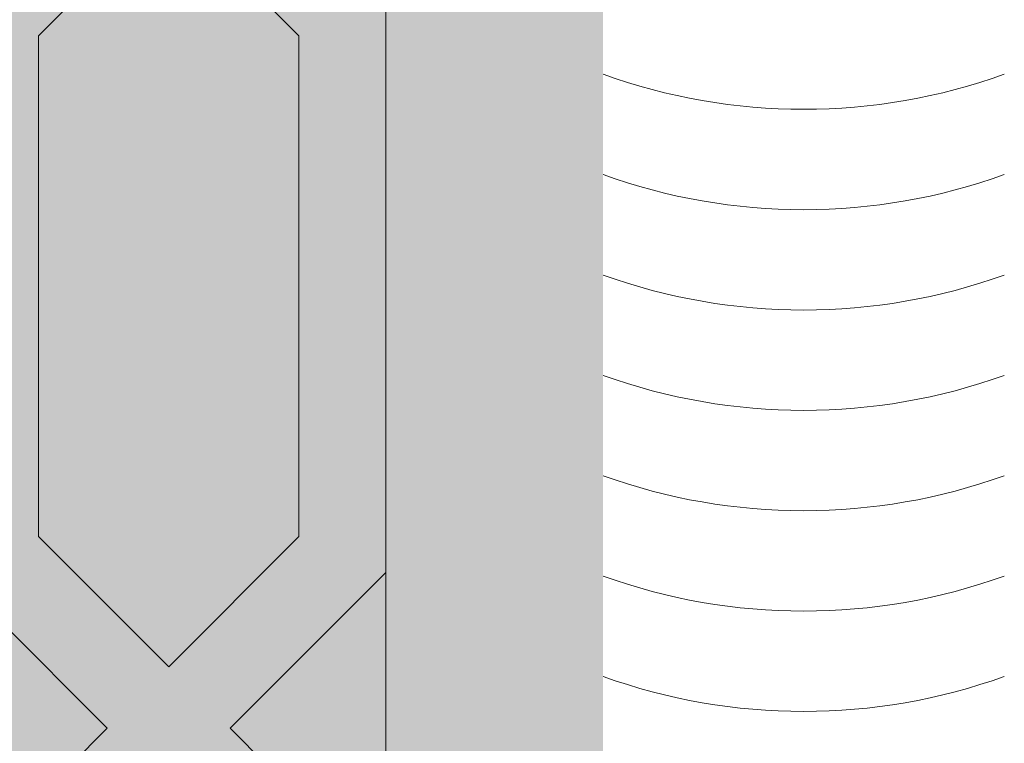
# Model space of a CAD drawing. Units: inches. Extents: x 844 to 2234, y 346 to 1084.
# Tile 38 of 93: x 1262.676 to 1265.567, y 699.229 to 701.353. Entities that reach past the tile are written whole.
import ezdxf

# ---------------------------------------------------------------- set-up
doc = ezdxf.new("R2010")
doc.units = ezdxf.units.IN
doc.header["$MEASUREMENT"] = 0
doc.layers.add('furniture', color=8, linetype='Continuous', lineweight=18)
doc.layers.add('RA-AP-01$0$INT', color=35, linetype='Continuous', lineweight=5)
doc.layers.add('RA-AP-01$0$FURN', color=3, linetype='Continuous')

# ---------------------------------------------------------------- blocks, each defined once
blk = doc.blocks.new('A$C18D01794')
at = {"layer": 'RA-AP-01$0$INT'}
h = blk.add_hatch(color=256, dxfattribs=at)
h.paths.add_polyline_path([(4.355206456958071, -6.156712009588037), (4.355206456958071, -8.056712009588038), (5.455206456958072, -8.056712009588038), (5.455206456958072, -6.156712009588037)])
h.paths.add_polyline_path([(4.405206456958072, -8.006712009588039), (4.405206456958072, -6.206712009588038), (5.405206456958072, -6.206712009588038), (5.405206456958072, -8.006712009588039)], flags=16)
h = blk.add_hatch(color=256, dxfattribs=at)
h.paths.add_polyline_path([(4.505206456958071, -7.585498806127123), (4.46934859260189, -7.549640941759413), (4.505206456958071, -7.513783077414768), (4.505206456958071, -7.381963272220687), (4.469348592616735, -7.346105407867824), (4.505206456958071, -7.310247543514964), (4.505206456958071, -7.178427738324996), (4.469348592586679, -7.142569873965138), (4.505206456952245, -7.106712009588038), (4.476922185709333, -7.106712009588038), (4.455206456960671, -7.128427738343681), (4.433490728198047, -7.106712009588038), (4.405206456946033, -7.106712009588036), (4.441064321339216, -7.142569873969684), (4.40520645695807, -7.178427738362358), (4.405206456958072, -7.310247543472698), (4.441064321364728, -7.346105407867826), (4.40520645695807, -7.381963272262947), (4.40520645695807, -7.513783077378263), (4.441064321354429, -7.549640941786153), (4.405206456958072, -7.585498806170974), (4.405206456958072, -7.717318611286652), (4.441064321333084, -7.753176475673194), (4.405206456958072, -7.789034340036673), (4.405206456958072, -8.006712009588039), (4.644348592588106, -8.006712009588039), (4.680206456964639, -7.970854145211967), (4.716064321341165, -8.006712009588039), (4.869348592586113, -8.006712009588039), (4.905206456964143, -7.970854145210465), (4.941064321342174, -8.006712009588039), (5.094348592587118, -8.006712009588037), (5.130206456963649, -7.970854145211967), (5.166064321340178, -8.006712009588039), (5.405206456958072, -8.006712009588039), (5.405206456958072, -7.789034340024526), (5.369348592595202, -7.753176475673196), (5.40520645695807, -7.717318611298797), (5.40520645695807, -7.585498806158829), (5.369348592573859, -7.549640941786151), (5.40520645695807, -7.51378307739041), (5.40520645695807, -7.381963272250803), (5.36934859256356, -7.346105407867824), (5.405206456958072, -7.310247543484846), (5.405206456958072, -7.178427738350217), (5.369348592589068, -7.142569873969682), (5.405206456982249, -7.106712009588038), (5.376922185730244, -7.106712009588038), (5.355206456967613, -7.128427738343679), (5.333490728218955, -7.10671200958804), (5.305206456976043, -7.106712009588042), (5.341064321341609, -7.142569873965136), (5.305206456958072, -7.178427738337141), (5.305206456958072, -7.310247543502816), (5.34106432131155, -7.346105407867824), (5.305206456958072, -7.381963272232832), (5.30520645695807, -7.513783077402624), (5.341064321326395, -7.549640941759413), (5.305206456958072, -7.585498806139263), (5.305206456958072, -7.717318611299605), (5.341064321347738, -7.753176475677737), (5.305206456958072, -7.78903434007894), (5.30520645695807, -7.906712009588039), (5.166064321336834, -7.906712009588039), (5.130206456963647, -7.942569873961684), (5.094348592590464, -7.906712009588039), (4.941064321338827, -7.906712009588041), (4.905206456964145, -7.942569873963183), (4.869348592589459, -7.906712009588039), (4.716064321337822, -7.906712009588041), (4.680206456964641, -7.942569873961684), (4.644348592591453, -7.906712009588039), (4.505206456958071, -7.906712009588039), (4.505206456958071, -7.789034340066795), (4.469348592580545, -7.753176475677738), (4.505206456958071, -7.717318611311748)])
h.paths.add_polyline_path([(4.485206456974132, -7.709034340046354), (4.45520645695909, -7.739034340051736), (4.425206456974128, -7.709034340057131), (4.425206456993394, -7.593783077384998), (4.45520645699153, -7.563783077396511), (4.485206456993396, -7.593783077408017)], flags=16)
h.paths.add_polyline_path([(4.455206456954537, -7.767318611299197), (4.485206456958242, -7.797318611312542), (4.48520645695951, -7.912569873958716), (4.45520645695415, -7.942569873954422), (4.425206456957888, -7.912569873967813), (4.425206456957888, -7.797318611286197)], flags=16)
h.paths.add_polyline_path([(4.455206456964794, -7.535498806149051), (4.42520645696469, -7.5054988061393), (4.425206456983954, -7.390247543486406), (4.455206456990734, -7.360247543489279), (4.485206456983953, -7.39024754349214), (4.485206456964687, -7.505498806158811)], flags=16)
h.paths.add_polyline_path([(4.499348592588947, -7.926712009585049), (4.636064321340932, -7.926712009585049), (4.666064321342317, -7.956712009586821), (4.636064321343707, -7.986712009585048), (4.499348592575121, -7.986712009585048), (4.469348592591685, -7.956712009591957)], flags=16)
h.paths.add_polyline_path([(4.425206456957888, -7.940854145195974), (4.471064321332215, -7.986712009585049), (4.425206456957888, -7.986712009585049)], flags=16)
h.paths.add_polyline_path([(4.455206456990734, -7.331963272246367), (4.425206456989053, -7.301963272254337), (4.425206456969784, -7.186712009596224), (4.455206456965226, -7.156712009591144), (4.485206456969787, -7.186712009586051), (4.485206456989053, -7.301963272238404)], flags=16)
h.paths.add_polyline_path([(4.72434859258714, -7.926712009586255), (4.861064321340141, -7.926712009586248), (4.891064321340324, -7.956712009586823), (4.861064321340513, -7.986712009586252), (4.724348592586768, -7.986712009586252), (4.694348592586956, -7.956712009586821)], flags=16)
h.paths.add_polyline_path([(4.919348592587961, -7.956712009586821), (4.949348592588145, -7.92671200958625), (5.08606432134115, -7.926712009586253), (5.116064321341327, -7.956712009586823), (5.086064321341519, -7.986712009586252), (4.949348592587774, -7.986712009586252)], flags=16)
h.paths.add_polyline_path([(5.144348592585967, -7.956712009586823), (5.174348592587358, -7.926712009585049), (5.311064321339338, -7.926712009585049), (5.3410643213366, -7.956712009591957), (5.311064321353163, -7.986712009585048), (5.174348592584576, -7.986712009585048)], flags=16)
h.paths.add_polyline_path([(5.32520645693489, -7.593783077408021), (5.355206456936755, -7.563783077396511), (5.385206456934894, -7.593783077384998), (5.38520645695416, -7.709034340057128), (5.355206456969194, -7.739034340051736), (5.325206456954153, -7.709034340046352)], flags=16)
h.paths.add_polyline_path([(5.325206456970042, -7.797318611312542), (5.355206456973747, -7.767318611299197), (5.385206456970398, -7.7973186112862), (5.385206456970398, -7.912569873967816), (5.355206456974136, -7.942569873954422), (5.325206456968778, -7.912569873958716)], flags=16)
h.paths.add_polyline_path([(5.325206456963599, -7.505498806158811), (5.325206456944333, -7.39024754349214), (5.355206456937552, -7.360247543489279), (5.385206456944332, -7.39024754348641), (5.385206456963596, -7.505498806139303), (5.355206456963492, -7.53549880614905)], flags=16)
h.paths.add_polyline_path([(5.32520645693923, -7.301963272238403), (5.3252064569585, -7.186712009586051), (5.355206456963062, -7.156712009591142), (5.3852064569585, -7.186712009596224), (5.385206456939234, -7.301963272254338), (5.355206456937552, -7.331963272246369)], flags=16)
h.paths.add_polyline_path([(5.339348592596071, -7.986712009585048), (5.385206456970398, -7.940854145195972), (5.385206456970396, -7.986712009585048)], flags=16)
h = blk.add_hatch(color=256, dxfattribs=at)
h.paths.add_polyline_path([(4.469348592586677, -7.142569873965136), (4.505206456958073, -7.178427738324996), (4.505206456958071, -7.106712009582215)])
h.paths.add_polyline_path([(4.455206456960671, -7.128427738343681), (4.476922185709333, -7.106712009588038), (4.433490728198045, -7.106712009588038)])
h.paths.add_polyline_path([(4.405206456958073, -7.178427738362358), (4.441064321339218, -7.142569873969684), (4.40520645695807, -7.106712009600073)])
h.paths.add_polyline_path([(4.425206456989053, -7.301963272254335), (4.455206456990736, -7.331963272246371), (4.485206456989055, -7.301963272238399), (4.48520645696979, -7.186712009586054), (4.455206456965227, -7.15671200959114), (4.425206456969784, -7.186712009596224)])
h.paths.add_polyline_path([(4.505206456958073, -7.381963272220689), (4.505206456958071, -7.310247543514961), (4.469348592616738, -7.346105407867826)])
h.paths.add_polyline_path([(4.425206456964688, -7.5054988061393), (4.455206456964794, -7.535498806149051), (4.485206456964689, -7.505498806158811), (4.485206456983951, -7.390247543492138), (4.455206456990736, -7.360247543489277), (4.425206456983956, -7.39024754348641)])
h.paths.add_polyline_path([(4.425206456974126, -7.709034340057128), (4.455206456959092, -7.739034340051736), (4.485206456974132, -7.709034340046356), (4.485206456993396, -7.593783077408017), (4.45520645699153, -7.563783077396511), (4.425206456993394, -7.593783077384999)])
h.paths.add_polyline_path([(4.46934859260189, -7.549640941759415), (4.505206456958071, -7.585498806127123), (4.505206456958073, -7.513783077414766)])
h.paths.add_polyline_path([(4.405206456958073, -7.585498806170972), (4.441064321354427, -7.549640941786151), (4.405206456958072, -7.513783077378263)])
h.paths.add_polyline_path([(4.405206456958072, -7.789034340036673), (4.441064321333084, -7.753176475673194), (4.405206456958072, -7.71731861128665)])
h.paths.add_polyline_path([(4.469348592580547, -7.75317647567774), (4.505206456958071, -7.789034340066795), (4.505206456958071, -7.717318611311744)])
h.paths.add_polyline_path([(4.425206456957888, -7.912569873967814), (4.45520645695415, -7.942569873954422), (4.485206456959507, -7.912569873958718), (4.48520645695824, -7.797318611312542), (4.455206456954537, -7.767318611299197), (4.425206456957888, -7.797318611286202)])
h.paths.add_polyline_path([(4.425206456957888, -7.986712009585049), (4.471064321332215, -7.986712009585049), (4.425206456957888, -7.940854145195972)])
h.paths.add_polyline_path([(4.499348592575121, -7.986712009585048), (4.636064321343707, -7.986712009585049), (4.666064321342317, -7.956712009586823), (4.636064321340932, -7.926712009585049), (4.499348592588945, -7.926712009585049), (4.469348592591685, -7.95671200959196)])
h.paths.add_polyline_path([(4.680206456964641, -7.942569873961684), (4.716064321337824, -7.906712009588039), (4.644348592591454, -7.906712009588039)])
h.paths.add_polyline_path([(4.644348592588108, -8.006712009588039), (4.716064321341167, -8.006712009588039), (4.680206456964637, -7.970854145211964)])
h.paths.add_polyline_path([(4.724348592586768, -7.98671200958625), (4.861064321340514, -7.986712009586252), (4.891064321340324, -7.956712009586819), (4.861064321340141, -7.92671200958625), (4.724348592587134, -7.926712009586255), (4.694348592586957, -7.956712009586821)])
h.paths.add_polyline_path([(4.905206456964143, -7.942569873963183), (4.941064321338827, -7.906712009588039), (4.869348592589457, -7.906712009588037)])
h.paths.add_polyline_path([(4.869348592586113, -8.006712009588039), (4.941064321342172, -8.006712009588037), (4.905206456964145, -7.970854145210463)])
h.paths.add_polyline_path([(4.949348592587774, -7.986712009586252), (5.086064321341521, -7.986712009586252), (5.116064321341329, -7.956712009586823), (5.08606432134115, -7.926712009586253), (4.949348592588145, -7.92671200958625), (4.919348592587961, -7.956712009586819)])
h.paths.add_polyline_path([(5.130206456963645, -7.942569873961684), (5.166064321336834, -7.906712009588039), (5.094348592590464, -7.906712009588039)])
h.paths.add_polyline_path([(5.094348592587119, -8.006712009588039), (5.166064321340178, -8.006712009588039), (5.130206456963651, -7.970854145211967)])
h.paths.add_polyline_path([(5.174348592584578, -7.986712009585048), (5.311064321353163, -7.986712009585048), (5.341064321336602, -7.956712009591958), (5.31106432133934, -7.926712009585049), (5.174348592587352, -7.926712009585049), (5.144348592585969, -7.956712009586823)])
h.paths.add_polyline_path([(5.325206456968778, -7.912569873958718), (5.355206456974136, -7.942569873954422), (5.385206456970396, -7.912569873967814), (5.385206456970396, -7.797318611286199), (5.355206456973747, -7.767318611299197), (5.325206456970044, -7.797318611312544)])
h.paths.add_polyline_path([(5.339348592596073, -7.986712009585048), (5.385206456970396, -7.986712009585049), (5.385206456970398, -7.94085414519597)])
h.paths.add_polyline_path([(5.325206456954155, -7.709034340046354), (5.355206456969194, -7.739034340051734), (5.38520645695416, -7.709034340057128), (5.385206456934896, -7.593783077384999), (5.355206456936758, -7.563783077396513), (5.325206456934888, -7.593783077408019)])
h.paths.add_polyline_path([(5.305206456958072, -7.789034340078938), (5.341064321347739, -7.753176475677738), (5.305206456958072, -7.717318611299605)])
h.paths.add_polyline_path([(5.369348592595204, -7.753176475673194), (5.40520645695807, -7.789034340024526), (5.405206456958072, -7.717318611298798)])
h.paths.add_polyline_path([(5.405206456958072, -7.585498806158831), (5.405206456958072, -7.513783077390407), (5.369348592573857, -7.549640941786151)])
h.paths.add_polyline_path([(5.305206456958072, -7.585498806139266), (5.341064321326393, -7.549640941759413), (5.305206456958072, -7.513783077402626)])
h.paths.add_polyline_path([(5.325206456963599, -7.50549880615881), (5.355206456963494, -7.535498806149055), (5.385206456963598, -7.505498806139302), (5.385206456944334, -7.390247543486411), (5.355206456937552, -7.360247543489279), (5.325206456944333, -7.39024754349214)])
h.paths.add_polyline_path([(5.305206456958072, -7.38196327223283), (5.341064321311551, -7.346105407867824), (5.305206456958072, -7.31024754350282)])
h.paths.add_polyline_path([(5.325206456939231, -7.301963272238404), (5.355206456937552, -7.331963272246369), (5.385206456939235, -7.301963272254335), (5.385206456958502, -7.186712009596224), (5.355206456963061, -7.156712009591142), (5.3252064569585, -7.186712009586051)])
h.paths.add_polyline_path([(5.404581768715993, -7.381338584008926, -0.001217816984214), (5.405206456958072, -7.381112009582329), (5.405206456958072, -7.310247543484846), (5.369348592563558, -7.346105407867826)])
h.paths.add_polyline_path([(5.36934859258907, -7.142569873969684), (5.40520645695807, -7.178427738350215), (5.405206456958072, -7.106712009612218)])
h.paths.add_polyline_path([(5.355206456967613, -7.128427738343683), (5.376922185730239, -7.106712009588038), (5.333490728218953, -7.10671200958804)])
h.paths.add_polyline_path([(5.30520645695807, -7.178427738337139), (5.341064321341609, -7.142569873965134), (5.305206456958074, -7.10671200957007)])
blk.add_hatch(color=256, dxfattribs=at).paths.add_polyline_path([(4.405206456958072, -7.381963272262946), (4.441064321364729, -7.346105407867824), (4.405206456958072, -7.310247543472702)])
for p, q in [((4.405206456987673, -7.310247543502303), (4.441064321369275, -7.346105407872371)), ((4.505206456987672, -7.31024754348536), (4.469348592616737, -7.346105407867824)), ((4.405206456987673, -7.381963272233345), (4.441064321369275, -7.346105407863277)), ((4.505206456987672, -7.381963272250288), (4.469348592616737, -7.346105407867824)), ((4.425206456983954, -7.39024754348641), (4.455206456990734, -7.360247543489279)), ((4.485206456983953, -7.39024754349214), (4.455206456990734, -7.360247543489279)), ((4.425206456983954, -7.39024754348641), (4.425206456964688, -7.5054988061393)), ((4.485206456983953, -7.39024754349214), (4.485206456964687, -7.505498806158811)), ((4.425206456964688, -7.5054988061393), (4.455206456964796, -7.535498806149051)), ((4.485206456964687, -7.505498806158811), (4.455206456964796, -7.535498806149051))]:
    blk.add_line(p, q, dxfattribs=at)
blk.add_lwpolyline([(5.405206456958072, -8.006712009588039), (4.405206456958072, -8.006712009588039), (4.405206456958072, -7.106712009588038)], dxfattribs=at)
for centre in [(4.309006456955496, -7.486364458281093), (4.309006456953905, -7.509464458285981), (4.309006456952086, -7.532564458284502), (4.309006456955041, -7.555664458280295), (4.309006456954814, -7.578764458284956), (4.309006456953222, -7.601864458283705), (4.309006456951631, -7.624964458285409)]:
    blk.add_arc(centre, 0.136414042854523, 70.20384312815696, 109.7961568705686, dxfattribs=at)
blk = doc.blocks.new('A$C5D2F253E')
at = {"layer": 'RA-AP-01$0$FURN', "xscale": -0.7999999999883585, "yscale": 0.7999999999883585, "zscale": 0.8, "rotation": 90}
blk.add_blockref('A$C18D01794', (-5.687757199772477, 4.75791982714071), dxfattribs=at)

msp = doc.modelspace()

# ---------------------------------------------------------------- block references
at = {"layer": 'furniture', "xscale": -15.94108302203742, "yscale": 15.94108302203742, "zscale": 15.94108302203742, "rotation": 270}
msp.add_blockref('A$C5D2F253E', (1244.08405109492, 696.2584716700112), dxfattribs=at)

doc.saveas('drawing.dxf')
